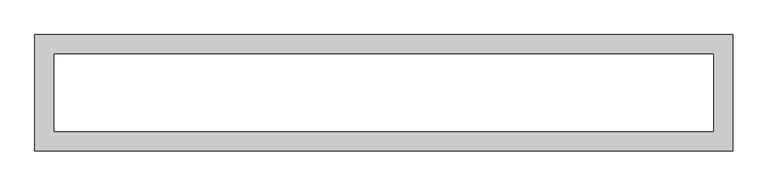
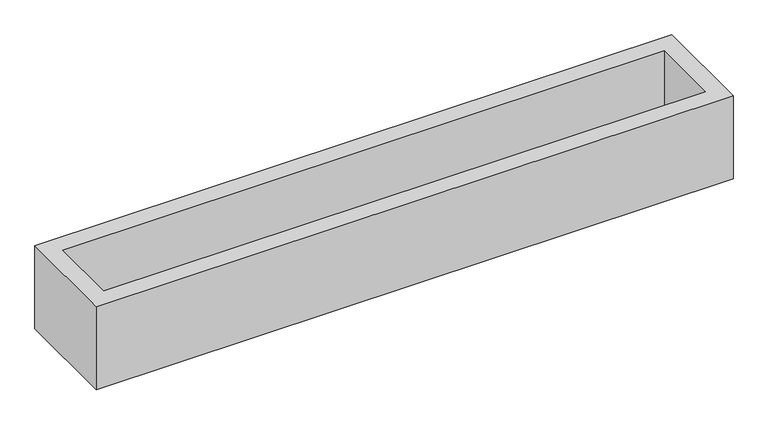
"""IFC4 building model written with IfcOpenShell, lengths in millimetres: proxy geometry."""

from ifc_helpers import new_model, si_unit, origin, origin_with_axes, place, context, project, spatial, polyline, outline, extrude, source, transform, mapped, element, save


def generic_models_4629e616(model_context):
    return source(origin(), model_context, "Body", "SweptSolid", [
        extrude(outline(polyline([(2430.835938, -6829.6142637), (2430.835938, -7744.0142637), (-3055.564062, -7744.0142637), (-3055.564062, -6829.6142637), (2430.835938, -6829.6142637)]), holes=[polyline([(2278.435938, -7591.6142637), (2278.435938, -6982.0142637), (-2903.164062, -6982.0142637), (-2903.164062, -7591.6142637), (2278.435938, -7591.6142637)])]), origin_with_axes(), (0.0, 0.0, 1.0), 757.4826469),
    ])


if __name__ == "__main__":
    model = new_model("IFC4")
    model_context = context("Model", 3, world=origin())
    ifc_project = project(units=[si_unit("LENGTHUNIT", "METRE", prefix="MILLI")], contexts=[model_context])
    site = spatial("IfcSite", under=ifc_project)
    building = spatial("IfcBuilding", under=site)
    placement = place(None, origin())
    generic_models_shape = generic_models_4629e616(model_context)
    element("IfcBuildingElementProxy", 1, Name="Generic Models", at=placement, inside=building, context=model_context, shape_type="MappedRepresentation", body=[
        mapped(generic_models_shape, transform((0.0, 0.0, 0.0), x_axis=(1.0, 0.0, 0.0), y_axis=(0.0, 1.0, 0.0), z_axis=(0.0, 0.0, 1.0))),
    ])
    save(model, "model.ifc")
